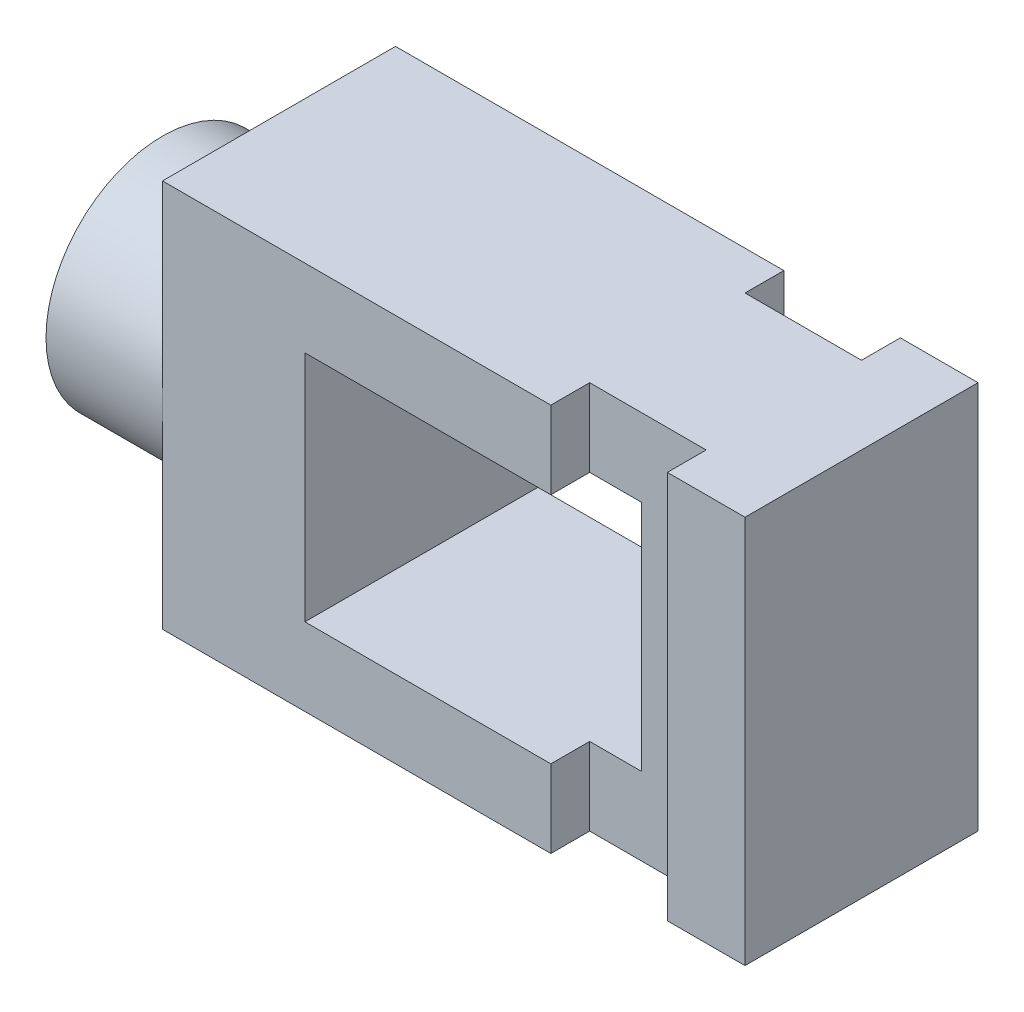
ISO-10303-21;
HEADER;
FILE_DESCRIPTION(('STEP AP214'),'2;1');
FILE_NAME('part.step','',(''),(''),'','','');
FILE_SCHEMA(('AUTOMOTIVE_DESIGN { 1 0 10303 214 1 1 1 1 }'));
ENDSEC;
DATA;
#1=APPLICATION_CONTEXT('core data for automotive mechanical design processes');
#2=APPLICATION_PROTOCOL_DEFINITION('international standard','automotive_design',2000,#1);
#3=PRODUCT_CONTEXT('',#1,'mechanical');
#4=PRODUCT('Part','Part','',(#3));
#5=PRODUCT_RELATED_PRODUCT_CATEGORY('part','',(#4));
#6=PRODUCT_DEFINITION_FORMATION('','',#4);
#7=PRODUCT_DEFINITION_CONTEXT('part definition',#1,'design');
#8=PRODUCT_DEFINITION('design','',#6,#7);
#9=PRODUCT_DEFINITION_SHAPE('','',#8);
#10=(LENGTH_UNIT() NAMED_UNIT(*) SI_UNIT(.MILLI.,.METRE.));
#11=(NAMED_UNIT(*) PLANE_ANGLE_UNIT() SI_UNIT($,.RADIAN.));
#12=(NAMED_UNIT(*) SI_UNIT($,.STERADIAN.) SOLID_ANGLE_UNIT());
#13=UNCERTAINTY_MEASURE_WITH_UNIT(LENGTH_MEASURE(1.E-05),#10,'distance_accuracy_value','');
#14=(GEOMETRIC_REPRESENTATION_CONTEXT(3) GLOBAL_UNCERTAINTY_ASSIGNED_CONTEXT((#13)) GLOBAL_UNIT_ASSIGNED_CONTEXT((#10,
#11,#12)) REPRESENTATION_CONTEXT('',''));
#15=CARTESIAN_POINT('',(0.,0.,0.));
#16=DIRECTION('',(0.,0.,1.));
#17=DIRECTION('',(1.,0.,0.));
#18=AXIS2_PLACEMENT_3D('',#15,#16,#17);
#19=CARTESIAN_POINT('',(0.,0.,36.));
#20=DIRECTION('',(0.,0.,-1.));
#21=DIRECTION('',(-1.,0.,0.));
#22=AXIS2_PLACEMENT_3D('',#19,#20,#21);
#23=PLANE('',#22);
#24=DIRECTION('',(1.,0.,0.));
#25=VECTOR('',#24,1.);
#26=CARTESIAN_POINT('',(-45.,-30.,36.));
#27=LINE('',#26,#25);
#28=CARTESIAN_POINT('',(-45.,-30.,36.));
#29=VERTEX_POINT('',#28);
#30=CARTESIAN_POINT('',(15.,-30.,36.));
#31=VERTEX_POINT('',#30);
#32=EDGE_CURVE('E314',#29,#31,#27,.T.);
#33=ORIENTED_EDGE('',*,*,#32,.T.);
#34=DIRECTION('',(0.,1.,0.));
#35=VECTOR('',#34,1.);
#36=CARTESIAN_POINT('',(15.,0.,36.));
#37=LINE('',#36,#35);
#38=CARTESIAN_POINT('',(15.,-18.,36.));
#39=VERTEX_POINT('',#38);
#40=EDGE_CURVE('E50',#31,#39,#37,.T.);
#41=ORIENTED_EDGE('',*,*,#40,.T.);
#42=DIRECTION('',(1.,0.,0.));
#43=VECTOR('',#42,1.);
#44=CARTESIAN_POINT('',(-23.,-18.,36.));
#45=LINE('',#44,#43);
#46=CARTESIAN_POINT('',(-23.,-18.,36.));
#47=VERTEX_POINT('',#46);
#48=EDGE_CURVE('E278',#47,#39,#45,.T.);
#49=ORIENTED_EDGE('',*,*,#48,.F.);
#50=DIRECTION('',(0.,-1.,0.));
#51=VECTOR('',#50,1.);
#52=CARTESIAN_POINT('',(-23.,-18.,36.));
#53=LINE('',#52,#51);
#54=CARTESIAN_POINT('',(-23.,18.,36.));
#55=VERTEX_POINT('',#54);
#56=EDGE_CURVE('E288',#55,#47,#53,.T.);
#57=ORIENTED_EDGE('',*,*,#56,.F.);
#58=DIRECTION('',(-1.,0.,0.));
#59=VECTOR('',#58,1.);
#60=CARTESIAN_POINT('',(-23.,18.,36.));
#61=LINE('',#60,#59);
#62=CARTESIAN_POINT('',(15.,18.,36.));
#63=VERTEX_POINT('',#62);
#64=EDGE_CURVE('E271',#63,#55,#61,.T.);
#65=ORIENTED_EDGE('',*,*,#64,.F.);
#66=DIRECTION('',(0.,-1.,0.));
#67=VECTOR('',#66,1.);
#68=CARTESIAN_POINT('',(15.,30.,36.));
#69=LINE('',#68,#67);
#70=CARTESIAN_POINT('',(15.,30.,36.));
#71=VERTEX_POINT('',#70);
#72=EDGE_CURVE('E213',#71,#63,#69,.T.);
#73=ORIENTED_EDGE('',*,*,#72,.F.);
#74=DIRECTION('',(-1.,0.,0.));
#75=VECTOR('',#74,1.);
#76=CARTESIAN_POINT('',(-45.,30.,36.));
#77=LINE('',#76,#75);
#78=CARTESIAN_POINT('',(-45.,30.,36.));
#79=VERTEX_POINT('',#78);
#80=EDGE_CURVE('E204',#71,#79,#77,.T.);
#81=ORIENTED_EDGE('',*,*,#80,.T.);
#82=DIRECTION('',(0.,-1.,0.));
#83=VECTOR('',#82,1.);
#84=CARTESIAN_POINT('',(-45.,-30.,36.));
#85=LINE('',#84,#83);
#86=CARTESIAN_POINT('',(-45.,0.,36.));
#87=VERTEX_POINT('',#86);
#88=EDGE_CURVE('E315',#79,#87,#85,.T.);
#89=ORIENTED_EDGE('',*,*,#88,.T.);
#90=EDGE_CURVE('E311',#87,#29,#85,.T.);
#91=ORIENTED_EDGE('',*,*,#90,.T.);
#92=EDGE_LOOP('',(#33,#41,#49,#57,#65,#73,#81,#89,#91));
#93=FACE_BOUND('',#92,.T.);
#94=ADVANCED_FACE('F39',(#93),#23,.F.);
#95=CARTESIAN_POINT('',(-45.,30.,36.));
#96=DIRECTION('',(0.,-1.,0.));
#97=DIRECTION('',(0.,0.,-1.));
#98=AXIS2_PLACEMENT_3D('',#95,#96,#97);
#99=PLANE('',#98);
#100=ORIENTED_EDGE('',*,*,#80,.F.);
#101=DIRECTION('',(0.,0.,-1.));
#102=VECTOR('',#101,1.);
#103=CARTESIAN_POINT('',(15.,30.,36.));
#104=LINE('',#103,#102);
#105=CARTESIAN_POINT('',(15.,30.,30.));
#106=VERTEX_POINT('',#105);
#107=EDGE_CURVE('E184',#71,#106,#104,.T.);
#108=ORIENTED_EDGE('',*,*,#107,.T.);
#109=DIRECTION('',(1.,0.,0.));
#110=VECTOR('',#109,1.);
#111=CARTESIAN_POINT('',(15.,30.,30.));
#112=LINE('',#111,#110);
#113=CARTESIAN_POINT('',(33.,30.,30.));
#114=VERTEX_POINT('',#113);
#115=EDGE_CURVE('E191',#106,#114,#112,.T.);
#116=ORIENTED_EDGE('',*,*,#115,.T.);
#117=DIRECTION('',(0.,0.,1.));
#118=VECTOR('',#117,1.);
#119=CARTESIAN_POINT('',(33.,30.,36.));
#120=LINE('',#119,#118);
#121=CARTESIAN_POINT('',(33.,30.,36.));
#122=VERTEX_POINT('',#121);
#123=EDGE_CURVE('E197',#114,#122,#120,.T.);
#124=ORIENTED_EDGE('',*,*,#123,.T.);
#125=CARTESIAN_POINT('',(45.,30.,36.));
#126=VERTEX_POINT('',#125);
#127=EDGE_CURVE('E308',#126,#122,#77,.T.);
#128=ORIENTED_EDGE('',*,*,#127,.F.);
#129=DIRECTION('',(0.,0.,-1.));
#130=VECTOR('',#129,1.);
#131=CARTESIAN_POINT('',(45.,30.,36.));
#132=LINE('',#131,#130);
#133=CARTESIAN_POINT('',(45.,30.,0.));
#134=VERTEX_POINT('',#133);
#135=EDGE_CURVE('E338',#126,#134,#132,.T.);
#136=ORIENTED_EDGE('',*,*,#135,.T.);
#137=DIRECTION('',(-1.,0.,0.));
#138=VECTOR('',#137,1.);
#139=CARTESIAN_POINT('',(-45.,30.,0.));
#140=LINE('',#139,#138);
#141=CARTESIAN_POINT('',(33.,30.,0.));
#142=VERTEX_POINT('',#141);
#143=EDGE_CURVE('E325',#134,#142,#140,.T.);
#144=ORIENTED_EDGE('',*,*,#143,.T.);
#145=DIRECTION('',(0.,0.,1.));
#146=VECTOR('',#145,1.);
#147=CARTESIAN_POINT('',(33.,30.,0.));
#148=LINE('',#147,#146);
#149=CARTESIAN_POINT('',(33.,30.,6.));
#150=VERTEX_POINT('',#149);
#151=EDGE_CURVE('E233',#142,#150,#148,.T.);
#152=ORIENTED_EDGE('',*,*,#151,.T.);
#153=DIRECTION('',(1.,0.,0.));
#154=VECTOR('',#153,1.);
#155=CARTESIAN_POINT('',(0.,30.,6.));
#156=LINE('',#155,#154);
#157=CARTESIAN_POINT('',(15.,30.,6.));
#158=VERTEX_POINT('',#157);
#159=EDGE_CURVE('E234',#158,#150,#156,.T.);
#160=ORIENTED_EDGE('',*,*,#159,.F.);
#161=DIRECTION('',(0.,0.,1.));
#162=VECTOR('',#161,1.);
#163=CARTESIAN_POINT('',(15.,30.,0.));
#164=LINE('',#163,#162);
#165=CARTESIAN_POINT('',(15.,30.,0.));
#166=VERTEX_POINT('',#165);
#167=EDGE_CURVE('E240',#166,#158,#164,.T.);
#168=ORIENTED_EDGE('',*,*,#167,.F.);
#169=CARTESIAN_POINT('',(-45.,30.,0.));
#170=VERTEX_POINT('',#169);
#171=EDGE_CURVE('E322',#166,#170,#140,.T.);
#172=ORIENTED_EDGE('',*,*,#171,.T.);
#173=DIRECTION('',(0.,0.,-1.));
#174=VECTOR('',#173,1.);
#175=CARTESIAN_POINT('',(-45.,30.,36.));
#176=LINE('',#175,#174);
#177=EDGE_CURVE('E340',#79,#170,#176,.T.);
#178=ORIENTED_EDGE('',*,*,#177,.F.);
#179=EDGE_LOOP('',(#100,#108,#116,#124,#128,#136,#144,#152,#160,#168,#172,#178));
#180=FACE_BOUND('',#179,.T.);
#181=ADVANCED_FACE('F203',(#180),#99,.F.);
#182=CARTESIAN_POINT('',(-45.,-30.,36.));
#183=DIRECTION('',(0.,1.,0.));
#184=DIRECTION('',(0.,0.,1.));
#185=AXIS2_PLACEMENT_3D('',#182,#183,#184);
#186=PLANE('',#185);
#187=DIRECTION('',(1.,0.,0.));
#188=VECTOR('',#187,1.);
#189=CARTESIAN_POINT('',(15.,-30.,30.));
#190=LINE('',#189,#188);
#191=CARTESIAN_POINT('',(15.,-30.,30.));
#192=VERTEX_POINT('',#191);
#193=CARTESIAN_POINT('',(33.,-30.,30.));
#194=VERTEX_POINT('',#193);
#195=EDGE_CURVE('E210',#192,#194,#190,.T.);
#196=ORIENTED_EDGE('',*,*,#195,.F.);
#197=DIRECTION('',(0.,0.,-1.));
#198=VECTOR('',#197,1.);
#199=CARTESIAN_POINT('',(15.,-30.,36.));
#200=LINE('',#199,#198);
#201=EDGE_CURVE('E212',#31,#192,#200,.T.);
#202=ORIENTED_EDGE('',*,*,#201,.F.);
#203=ORIENTED_EDGE('',*,*,#32,.F.);
#204=DIRECTION('',(0.,0.,-1.));
#205=VECTOR('',#204,1.);
#206=CARTESIAN_POINT('',(-45.,-30.,36.));
#207=LINE('',#206,#205);
#208=CARTESIAN_POINT('',(-45.,-30.,0.));
#209=VERTEX_POINT('',#208);
#210=EDGE_CURVE('E332',#29,#209,#207,.T.);
#211=ORIENTED_EDGE('',*,*,#210,.T.);
#212=DIRECTION('',(1.,0.,0.));
#213=VECTOR('',#212,1.);
#214=CARTESIAN_POINT('',(-45.,-30.,0.));
#215=LINE('',#214,#213);
#216=CARTESIAN_POINT('',(15.,-30.,0.));
#217=VERTEX_POINT('',#216);
#218=EDGE_CURVE('E310',#209,#217,#215,.T.);
#219=ORIENTED_EDGE('',*,*,#218,.T.);
#220=DIRECTION('',(0.,0.,1.));
#221=VECTOR('',#220,1.);
#222=CARTESIAN_POINT('',(15.,-30.,0.));
#223=LINE('',#222,#221);
#224=CARTESIAN_POINT('',(15.,-30.,6.));
#225=VERTEX_POINT('',#224);
#226=EDGE_CURVE('E232',#217,#225,#223,.T.);
#227=ORIENTED_EDGE('',*,*,#226,.T.);
#228=DIRECTION('',(1.,0.,0.));
#229=VECTOR('',#228,1.);
#230=CARTESIAN_POINT('',(0.,-30.,6.));
#231=LINE('',#230,#229);
#232=CARTESIAN_POINT('',(33.,-30.,6.));
#233=VERTEX_POINT('',#232);
#234=EDGE_CURVE('E245',#225,#233,#231,.T.);
#235=ORIENTED_EDGE('',*,*,#234,.T.);
#236=DIRECTION('',(0.,0.,1.));
#237=VECTOR('',#236,1.);
#238=CARTESIAN_POINT('',(33.,-30.,0.));
#239=LINE('',#238,#237);
#240=CARTESIAN_POINT('',(33.,-30.,0.));
#241=VERTEX_POINT('',#240);
#242=EDGE_CURVE('E229',#241,#233,#239,.T.);
#243=ORIENTED_EDGE('',*,*,#242,.F.);
#244=CARTESIAN_POINT('',(45.,-30.,0.));
#245=VERTEX_POINT('',#244);
#246=EDGE_CURVE('E329',#241,#245,#215,.T.);
#247=ORIENTED_EDGE('',*,*,#246,.T.);
#248=DIRECTION('',(0.,0.,-1.));
#249=VECTOR('',#248,1.);
#250=CARTESIAN_POINT('',(45.,-30.,36.));
#251=LINE('',#250,#249);
#252=CARTESIAN_POINT('',(45.,-30.,36.));
#253=VERTEX_POINT('',#252);
#254=EDGE_CURVE('E319',#253,#245,#251,.T.);
#255=ORIENTED_EDGE('',*,*,#254,.F.);
#256=CARTESIAN_POINT('',(33.,-30.,36.));
#257=VERTEX_POINT('',#256);
#258=EDGE_CURVE('E313',#257,#253,#27,.T.);
#259=ORIENTED_EDGE('',*,*,#258,.F.);
#260=DIRECTION('',(0.,0.,1.));
#261=VECTOR('',#260,1.);
#262=CARTESIAN_POINT('',(33.,-30.,36.));
#263=LINE('',#262,#261);
#264=EDGE_CURVE('E53',#194,#257,#263,.T.);
#265=ORIENTED_EDGE('',*,*,#264,.F.);
#266=EDGE_LOOP('',(#196,#202,#203,#211,#219,#227,#235,#243,#247,#255,#259,#265));
#267=FACE_BOUND('',#266,.T.);
#268=ADVANCED_FACE('F372',(#267),#186,.F.);
#269=CARTESIAN_POINT('',(0.,0.,0.));
#270=DIRECTION('',(0.,0.,-1.));
#271=DIRECTION('',(-1.,0.,0.));
#272=AXIS2_PLACEMENT_3D('',#269,#270,#271);
#273=PLANE('',#272);
#274=ORIENTED_EDGE('',*,*,#171,.F.);
#275=DIRECTION('',(0.,-1.,0.));
#276=VECTOR('',#275,1.);
#277=CARTESIAN_POINT('',(15.,30.,0.));
#278=LINE('',#277,#276);
#279=CARTESIAN_POINT('',(15.,18.,0.));
#280=VERTEX_POINT('',#279);
#281=EDGE_CURVE('E250',#166,#280,#278,.T.);
#282=ORIENTED_EDGE('',*,*,#281,.T.);
#283=DIRECTION('',(-1.,0.,0.));
#284=VECTOR('',#283,1.);
#285=CARTESIAN_POINT('',(-23.,18.,0.));
#286=LINE('',#285,#284);
#287=CARTESIAN_POINT('',(-23.,18.,0.));
#288=VERTEX_POINT('',#287);
#289=EDGE_CURVE('E280',#280,#288,#286,.T.);
#290=ORIENTED_EDGE('',*,*,#289,.T.);
#291=DIRECTION('',(0.,-1.,0.));
#292=VECTOR('',#291,1.);
#293=CARTESIAN_POINT('',(-23.,-18.,0.));
#294=LINE('',#293,#292);
#295=CARTESIAN_POINT('',(-23.,-18.,0.));
#296=VERTEX_POINT('',#295);
#297=EDGE_CURVE('E276',#288,#296,#294,.T.);
#298=ORIENTED_EDGE('',*,*,#297,.T.);
#299=DIRECTION('',(1.,0.,0.));
#300=VECTOR('',#299,1.);
#301=CARTESIAN_POINT('',(-23.,-18.,0.));
#302=LINE('',#301,#300);
#303=CARTESIAN_POINT('',(15.,-18.,0.));
#304=VERTEX_POINT('',#303);
#305=EDGE_CURVE('E281',#296,#304,#302,.T.);
#306=ORIENTED_EDGE('',*,*,#305,.T.);
#307=EDGE_CURVE('E249',#304,#217,#278,.T.);
#308=ORIENTED_EDGE('',*,*,#307,.T.);
#309=ORIENTED_EDGE('',*,*,#218,.F.);
#310=DIRECTION('',(0.,-1.,0.));
#311=VECTOR('',#310,1.);
#312=CARTESIAN_POINT('',(-45.,-30.,0.));
#313=LINE('',#312,#311);
#314=CARTESIAN_POINT('',(-45.,0.,0.));
#315=VERTEX_POINT('',#314);
#316=EDGE_CURVE('E323',#315,#209,#313,.T.);
#317=ORIENTED_EDGE('',*,*,#316,.F.);
#318=EDGE_CURVE('E328',#170,#315,#313,.T.);
#319=ORIENTED_EDGE('',*,*,#318,.F.);
#320=EDGE_LOOP('',(#274,#282,#290,#298,#306,#308,#309,#317,#319));
#321=FACE_BOUND('',#320,.T.);
#322=ADVANCED_FACE('F405',(#321),#273,.T.);
#323=CARTESIAN_POINT('',(23.,-18.,0.));
#324=DIRECTION('',(1.,0.,0.));
#325=DIRECTION('',(0.,0.,-1.));
#326=AXIS2_PLACEMENT_3D('',#323,#324,#325);
#327=PLANE('',#326);
#328=DIRECTION('',(0.,0.,1.));
#329=VECTOR('',#328,1.);
#330=CARTESIAN_POINT('',(23.,-18.,0.));
#331=LINE('',#330,#329);
#332=CARTESIAN_POINT('',(23.,-18.,6.));
#333=VERTEX_POINT('',#332);
#334=CARTESIAN_POINT('',(23.,-18.,30.));
#335=VERTEX_POINT('',#334);
#336=EDGE_CURVE('E291',#333,#335,#331,.T.);
#337=ORIENTED_EDGE('',*,*,#336,.T.);
#338=DIRECTION('',(0.,1.,0.));
#339=VECTOR('',#338,1.);
#340=CARTESIAN_POINT('',(23.,-18.,30.));
#341=LINE('',#340,#339);
#342=CARTESIAN_POINT('',(23.,18.,30.));
#343=VERTEX_POINT('',#342);
#344=EDGE_CURVE('E222',#335,#343,#341,.T.);
#345=ORIENTED_EDGE('',*,*,#344,.T.);
#346=DIRECTION('',(0.,0.,1.));
#347=VECTOR('',#346,1.);
#348=CARTESIAN_POINT('',(23.,18.,0.));
#349=LINE('',#348,#347);
#350=CARTESIAN_POINT('',(23.,18.,6.));
#351=VERTEX_POINT('',#350);
#352=EDGE_CURVE('E286',#351,#343,#349,.T.);
#353=ORIENTED_EDGE('',*,*,#352,.F.);
#354=DIRECTION('',(0.,1.,0.));
#355=VECTOR('',#354,1.);
#356=CARTESIAN_POINT('',(23.,-18.,6.));
#357=LINE('',#356,#355);
#358=EDGE_CURVE('E65',#333,#351,#357,.T.);
#359=ORIENTED_EDGE('',*,*,#358,.F.);
#360=EDGE_LOOP('',(#337,#345,#353,#359));
#361=FACE_BOUND('',#360,.T.);
#362=ADVANCED_FACE('F370',(#361),#327,.F.);
#363=CARTESIAN_POINT('',(-23.,-18.,0.));
#364=DIRECTION('',(0.,-1.,0.));
#365=DIRECTION('',(0.,0.,-1.));
#366=AXIS2_PLACEMENT_3D('',#363,#364,#365);
#367=PLANE('',#366);
#368=ORIENTED_EDGE('',*,*,#48,.T.);
#369=DIRECTION('',(0.,0.,-1.));
#370=VECTOR('',#369,1.);
#371=CARTESIAN_POINT('',(15.,-18.,0.));
#372=LINE('',#371,#370);
#373=CARTESIAN_POINT('',(15.,-18.,30.));
#374=VERTEX_POINT('',#373);
#375=EDGE_CURVE('E221',#39,#374,#372,.T.);
#376=ORIENTED_EDGE('',*,*,#375,.T.);
#377=DIRECTION('',(1.,0.,0.));
#378=VECTOR('',#377,1.);
#379=CARTESIAN_POINT('',(-23.,-18.,30.));
#380=LINE('',#379,#378);
#381=EDGE_CURVE('E227',#374,#335,#380,.T.);
#382=ORIENTED_EDGE('',*,*,#381,.T.);
#383=ORIENTED_EDGE('',*,*,#336,.F.);
#384=DIRECTION('',(1.,0.,0.));
#385=VECTOR('',#384,1.);
#386=CARTESIAN_POINT('',(-23.,-18.,6.));
#387=LINE('',#386,#385);
#388=CARTESIAN_POINT('',(15.,-18.,6.));
#389=VERTEX_POINT('',#388);
#390=EDGE_CURVE('E256',#389,#333,#387,.T.);
#391=ORIENTED_EDGE('',*,*,#390,.F.);
#392=DIRECTION('',(0.,0.,1.));
#393=VECTOR('',#392,1.);
#394=CARTESIAN_POINT('',(15.,-18.,0.));
#395=LINE('',#394,#393);
#396=EDGE_CURVE('E263',#304,#389,#395,.T.);
#397=ORIENTED_EDGE('',*,*,#396,.F.);
#398=ORIENTED_EDGE('',*,*,#305,.F.);
#399=DIRECTION('',(0.,0.,1.));
#400=VECTOR('',#399,1.);
#401=CARTESIAN_POINT('',(-23.,-18.,0.));
#402=LINE('',#401,#400);
#403=EDGE_CURVE('E300',#296,#47,#402,.T.);
#404=ORIENTED_EDGE('',*,*,#403,.T.);
#405=EDGE_LOOP('',(#368,#376,#382,#383,#391,#397,#398,#404));
#406=FACE_BOUND('',#405,.T.);
#407=ADVANCED_FACE('F352',(#406),#367,.F.);
#408=CARTESIAN_POINT('',(-23.,18.,0.));
#409=DIRECTION('',(0.,1.,0.));
#410=DIRECTION('',(0.,0.,1.));
#411=AXIS2_PLACEMENT_3D('',#408,#409,#410);
#412=PLANE('',#411);
#413=DIRECTION('',(-1.,0.,0.));
#414=VECTOR('',#413,1.);
#415=CARTESIAN_POINT('',(-23.,18.,30.));
#416=LINE('',#415,#414);
#417=CARTESIAN_POINT('',(15.,18.,30.));
#418=VERTEX_POINT('',#417);
#419=EDGE_CURVE('E11',#343,#418,#416,.T.);
#420=ORIENTED_EDGE('',*,*,#419,.T.);
#421=DIRECTION('',(0.,0.,1.));
#422=VECTOR('',#421,1.);
#423=CARTESIAN_POINT('',(15.,18.,0.));
#424=LINE('',#423,#422);
#425=EDGE_CURVE('E189',#418,#63,#424,.T.);
#426=ORIENTED_EDGE('',*,*,#425,.T.);
#427=ORIENTED_EDGE('',*,*,#64,.T.);
#428=DIRECTION('',(0.,0.,1.));
#429=VECTOR('',#428,1.);
#430=CARTESIAN_POINT('',(-23.,18.,0.));
#431=LINE('',#430,#429);
#432=EDGE_CURVE('E299',#288,#55,#431,.T.);
#433=ORIENTED_EDGE('',*,*,#432,.F.);
#434=ORIENTED_EDGE('',*,*,#289,.F.);
#435=DIRECTION('',(0.,0.,-1.));
#436=VECTOR('',#435,1.);
#437=CARTESIAN_POINT('',(15.,18.,0.));
#438=LINE('',#437,#436);
#439=CARTESIAN_POINT('',(15.,18.,6.));
#440=VERTEX_POINT('',#439);
#441=EDGE_CURVE('E343',#440,#280,#438,.T.);
#442=ORIENTED_EDGE('',*,*,#441,.F.);
#443=DIRECTION('',(-1.,0.,0.));
#444=VECTOR('',#443,1.);
#445=CARTESIAN_POINT('',(-23.,18.,6.));
#446=LINE('',#445,#444);
#447=EDGE_CURVE('E344',#351,#440,#446,.T.);
#448=ORIENTED_EDGE('',*,*,#447,.F.);
#449=ORIENTED_EDGE('',*,*,#352,.T.);
#450=EDGE_LOOP('',(#420,#426,#427,#433,#434,#442,#448,#449));
#451=FACE_BOUND('',#450,.T.);
#452=ADVANCED_FACE('F361',(#451),#412,.F.);
#453=CARTESIAN_POINT('',(-45.,-30.,36.));
#454=DIRECTION('',(1.,0.,0.));
#455=DIRECTION('',(0.,0.,-1.));
#456=AXIS2_PLACEMENT_3D('',#453,#454,#455);
#457=PLANE('',#456);
#458=CARTESIAN_POINT('',(-45.,0.,18.));
#459=DIRECTION('',(-1.,0.,0.));
#460=DIRECTION('',(0.,0.,1.));
#461=AXIS2_PLACEMENT_3D('',#458,#459,#460);
#462=CIRCLE('',#461,18.);
#463=EDGE_CURVE('E270',#87,#315,#462,.T.);
#464=ORIENTED_EDGE('',*,*,#463,.F.);
#465=ORIENTED_EDGE('',*,*,#88,.F.);
#466=ORIENTED_EDGE('',*,*,#177,.T.);
#467=ORIENTED_EDGE('',*,*,#318,.T.);
#468=EDGE_LOOP('',(#464,#465,#466,#467));
#469=FACE_BOUND('',#468,.T.);
#470=ADVANCED_FACE('F410',(#469),#457,.F.);
#471=CARTESIAN_POINT('',(45.,-30.,36.));
#472=DIRECTION('',(-1.,0.,0.));
#473=DIRECTION('',(0.,0.,1.));
#474=AXIS2_PLACEMENT_3D('',#471,#472,#473);
#475=PLANE('',#474);
#476=DIRECTION('',(0.,1.,0.));
#477=VECTOR('',#476,1.);
#478=CARTESIAN_POINT('',(45.,-30.,0.));
#479=LINE('',#478,#477);
#480=EDGE_CURVE('E298',#245,#134,#479,.T.);
#481=ORIENTED_EDGE('',*,*,#480,.T.);
#482=ORIENTED_EDGE('',*,*,#135,.F.);
#483=DIRECTION('',(0.,1.,0.));
#484=VECTOR('',#483,1.);
#485=CARTESIAN_POINT('',(45.,-30.,36.));
#486=LINE('',#485,#484);
#487=EDGE_CURVE('E302',#253,#126,#486,.T.);
#488=ORIENTED_EDGE('',*,*,#487,.F.);
#489=ORIENTED_EDGE('',*,*,#254,.T.);
#490=EDGE_LOOP('',(#481,#482,#488,#489));
#491=FACE_BOUND('',#490,.T.);
#492=ADVANCED_FACE('F41',(#491),#475,.F.);
#493=EDGE_CURVE('E277',#315,#87,#462,.T.);
#494=ORIENTED_EDGE('',*,*,#493,.F.);
#495=ORIENTED_EDGE('',*,*,#316,.T.);
#496=ORIENTED_EDGE('',*,*,#210,.F.);
#497=ORIENTED_EDGE('',*,*,#90,.F.);
#498=EDGE_LOOP('',(#494,#495,#496,#497));
#499=FACE_BOUND('',#498,.T.);
#500=ADVANCED_FACE('F414',(#499),#457,.F.);
#501=ORIENTED_EDGE('',*,*,#127,.T.);
#502=DIRECTION('',(0.,-1.,0.));
#503=VECTOR('',#502,1.);
#504=CARTESIAN_POINT('',(33.,30.,36.));
#505=LINE('',#504,#503);
#506=EDGE_CURVE('E220',#122,#257,#505,.T.);
#507=ORIENTED_EDGE('',*,*,#506,.T.);
#508=ORIENTED_EDGE('',*,*,#258,.T.);
#509=ORIENTED_EDGE('',*,*,#487,.T.);
#510=EDGE_LOOP('',(#501,#507,#508,#509));
#511=FACE_BOUND('',#510,.T.);
#512=ADVANCED_FACE('F378',(#511),#23,.F.);
#513=DIRECTION('',(0.,-1.,0.));
#514=VECTOR('',#513,1.);
#515=CARTESIAN_POINT('',(33.,30.,0.));
#516=LINE('',#515,#514);
#517=EDGE_CURVE('E237',#142,#241,#516,.T.);
#518=ORIENTED_EDGE('',*,*,#517,.F.);
#519=ORIENTED_EDGE('',*,*,#143,.F.);
#520=ORIENTED_EDGE('',*,*,#480,.F.);
#521=ORIENTED_EDGE('',*,*,#246,.F.);
#522=EDGE_LOOP('',(#518,#519,#520,#521));
#523=FACE_BOUND('',#522,.T.);
#524=ADVANCED_FACE('F390',(#523),#273,.T.);
#525=CARTESIAN_POINT('',(-23.,-18.,0.));
#526=DIRECTION('',(-1.,0.,0.));
#527=DIRECTION('',(0.,0.,1.));
#528=AXIS2_PLACEMENT_3D('',#525,#526,#527);
#529=PLANE('',#528);
#530=ORIENTED_EDGE('',*,*,#56,.T.);
#531=ORIENTED_EDGE('',*,*,#403,.F.);
#532=ORIENTED_EDGE('',*,*,#297,.F.);
#533=ORIENTED_EDGE('',*,*,#432,.T.);
#534=EDGE_LOOP('',(#530,#531,#532,#533));
#535=FACE_BOUND('',#534,.T.);
#536=ADVANCED_FACE('F360',(#535),#529,.F.);
#537=CARTESIAN_POINT('',(-63.,0.,18.));
#538=DIRECTION('',(1.,0.,0.));
#539=DIRECTION('',(0.,0.,-1.));
#540=AXIS2_PLACEMENT_3D('',#537,#538,#539);
#541=CYLINDRICAL_SURFACE('',#540,18.);
#542=CARTESIAN_POINT('',(-63.,0.,18.));
#543=DIRECTION('',(-1.,0.,0.));
#544=DIRECTION('',(0.,0.,1.));
#545=AXIS2_PLACEMENT_3D('',#542,#543,#544);
#546=CIRCLE('',#545,18.);
#547=CARTESIAN_POINT('',(-63.,0.,36.));
#548=VERTEX_POINT('',#547);
#549=EDGE_CURVE('E269',#548,#548,#546,.T.);
#550=ORIENTED_EDGE('',*,*,#549,.F.);
#551=EDGE_LOOP('',(#550));
#552=FACE_BOUND('',#551,.T.);
#553=ORIENTED_EDGE('',*,*,#463,.T.);
#554=ORIENTED_EDGE('',*,*,#493,.T.);
#555=EDGE_LOOP('',(#553,#554));
#556=FACE_BOUND('',#555,.T.);
#557=ADVANCED_FACE('F413',(#552,#556),#541,.T.);
#558=CARTESIAN_POINT('',(-63.,0.,18.));
#559=DIRECTION('',(-1.,0.,0.));
#560=DIRECTION('',(0.,0.,1.));
#561=AXIS2_PLACEMENT_3D('',#558,#559,#560);
#562=PLANE('',#561);
#563=CARTESIAN_POINT('',(-63.,0.,18.));
#564=DIRECTION('',(-1.,0.,0.));
#565=DIRECTION('',(0.,0.,1.));
#566=AXIS2_PLACEMENT_3D('',#563,#564,#565);
#567=CIRCLE('',#566,5.);
#568=CARTESIAN_POINT('',(-63.,0.,23.));
#569=VERTEX_POINT('',#568);
#570=EDGE_CURVE('E261',#569,#569,#567,.T.);
#571=ORIENTED_EDGE('',*,*,#570,.F.);
#572=EDGE_LOOP('',(#571));
#573=FACE_BOUND('',#572,.T.);
#574=ORIENTED_EDGE('',*,*,#549,.T.);
#575=EDGE_LOOP('',(#574));
#576=FACE_BOUND('',#575,.T.);
#577=ADVANCED_FACE('F543',(#573,#576),#562,.T.);
#578=CARTESIAN_POINT('',(-45.,0.,18.));
#579=DIRECTION('',(-1.,0.,0.));
#580=DIRECTION('',(0.,0.,1.));
#581=AXIS2_PLACEMENT_3D('',#578,#579,#580);
#582=CYLINDRICAL_SURFACE('',#581,5.);
#583=CARTESIAN_POINT('',(-45.,0.,18.));
#584=DIRECTION('',(-1.,0.,0.));
#585=DIRECTION('',(0.,0.,1.));
#586=AXIS2_PLACEMENT_3D('',#583,#584,#585);
#587=CIRCLE('',#586,5.);
#588=CARTESIAN_POINT('',(-45.,0.,23.));
#589=VERTEX_POINT('',#588);
#590=EDGE_CURVE('E264',#589,#589,#587,.T.);
#591=ORIENTED_EDGE('',*,*,#590,.F.);
#592=EDGE_LOOP('',(#591));
#593=FACE_BOUND('',#592,.T.);
#594=ORIENTED_EDGE('',*,*,#570,.T.);
#595=EDGE_LOOP('',(#594));
#596=FACE_BOUND('',#595,.T.);
#597=ADVANCED_FACE('F426',(#593,#596),#582,.F.);
#598=CARTESIAN_POINT('',(-45.,0.,18.));
#599=DIRECTION('',(-1.,0.,0.));
#600=DIRECTION('',(0.,0.,1.));
#601=AXIS2_PLACEMENT_3D('',#598,#599,#600);
#602=PLANE('',#601);
#603=ORIENTED_EDGE('',*,*,#590,.T.);
#604=EDGE_LOOP('',(#603));
#605=FACE_BOUND('',#604,.T.);
#606=ADVANCED_FACE('F423',(#605),#602,.T.);
#607=CARTESIAN_POINT('',(15.,30.,0.));
#608=DIRECTION('',(1.,0.,0.));
#609=DIRECTION('',(0.,0.,-1.));
#610=AXIS2_PLACEMENT_3D('',#607,#608,#609);
#611=PLANE('',#610);
#612=ORIENTED_EDGE('',*,*,#396,.T.);
#613=DIRECTION('',(0.,-1.,0.));
#614=VECTOR('',#613,1.);
#615=CARTESIAN_POINT('',(15.,30.,6.));
#616=LINE('',#615,#614);
#617=EDGE_CURVE('E251',#389,#225,#616,.T.);
#618=ORIENTED_EDGE('',*,*,#617,.T.);
#619=ORIENTED_EDGE('',*,*,#226,.F.);
#620=ORIENTED_EDGE('',*,*,#307,.F.);
#621=EDGE_LOOP('',(#612,#618,#619,#620));
#622=FACE_BOUND('',#621,.T.);
#623=ADVANCED_FACE('F418',(#622),#611,.T.);
#624=ORIENTED_EDGE('',*,*,#441,.T.);
#625=ORIENTED_EDGE('',*,*,#281,.F.);
#626=ORIENTED_EDGE('',*,*,#167,.T.);
#627=EDGE_CURVE('E252',#158,#440,#616,.T.);
#628=ORIENTED_EDGE('',*,*,#627,.T.);
#629=EDGE_LOOP('',(#624,#625,#626,#628));
#630=FACE_BOUND('',#629,.T.);
#631=ADVANCED_FACE('F419',(#630),#611,.T.);
#632=CARTESIAN_POINT('',(0.,30.,6.));
#633=DIRECTION('',(0.,0.,-1.));
#634=DIRECTION('',(-1.,0.,0.));
#635=AXIS2_PLACEMENT_3D('',#632,#633,#634);
#636=PLANE('',#635);
#637=ORIENTED_EDGE('',*,*,#390,.T.);
#638=ORIENTED_EDGE('',*,*,#358,.T.);
#639=ORIENTED_EDGE('',*,*,#447,.T.);
#640=ORIENTED_EDGE('',*,*,#627,.F.);
#641=ORIENTED_EDGE('',*,*,#159,.T.);
#642=DIRECTION('',(0.,-1.,0.));
#643=VECTOR('',#642,1.);
#644=CARTESIAN_POINT('',(33.,30.,6.));
#645=LINE('',#644,#643);
#646=EDGE_CURVE('E253',#150,#233,#645,.T.);
#647=ORIENTED_EDGE('',*,*,#646,.T.);
#648=ORIENTED_EDGE('',*,*,#234,.F.);
#649=ORIENTED_EDGE('',*,*,#617,.F.);
#650=EDGE_LOOP('',(#637,#638,#639,#640,#641,#647,#648,#649));
#651=FACE_BOUND('',#650,.T.);
#652=ADVANCED_FACE('F394',(#651),#636,.T.);
#653=CARTESIAN_POINT('',(33.,30.,0.));
#654=DIRECTION('',(1.,0.,0.));
#655=DIRECTION('',(0.,0.,-1.));
#656=AXIS2_PLACEMENT_3D('',#653,#654,#655);
#657=PLANE('',#656);
#658=ORIENTED_EDGE('',*,*,#242,.T.);
#659=ORIENTED_EDGE('',*,*,#646,.F.);
#660=ORIENTED_EDGE('',*,*,#151,.F.);
#661=ORIENTED_EDGE('',*,*,#517,.T.);
#662=EDGE_LOOP('',(#658,#659,#660,#661));
#663=FACE_BOUND('',#662,.T.);
#664=ADVANCED_FACE('F388',(#663),#657,.F.);
#665=CARTESIAN_POINT('',(15.,30.,30.));
#666=DIRECTION('',(0.,0.,-1.));
#667=DIRECTION('',(-1.,0.,0.));
#668=AXIS2_PLACEMENT_3D('',#665,#666,#667);
#669=PLANE('',#668);
#670=DIRECTION('',(0.,-1.,0.));
#671=VECTOR('',#670,1.);
#672=CARTESIAN_POINT('',(15.,30.,30.));
#673=LINE('',#672,#671);
#674=EDGE_CURVE('E192',#374,#192,#673,.T.);
#675=ORIENTED_EDGE('',*,*,#674,.T.);
#676=ORIENTED_EDGE('',*,*,#195,.T.);
#677=DIRECTION('',(0.,-1.,0.));
#678=VECTOR('',#677,1.);
#679=CARTESIAN_POINT('',(33.,30.,30.));
#680=LINE('',#679,#678);
#681=EDGE_CURVE('E188',#114,#194,#680,.T.);
#682=ORIENTED_EDGE('',*,*,#681,.F.);
#683=ORIENTED_EDGE('',*,*,#115,.F.);
#684=EDGE_CURVE('E181',#106,#418,#673,.T.);
#685=ORIENTED_EDGE('',*,*,#684,.T.);
#686=ORIENTED_EDGE('',*,*,#419,.F.);
#687=ORIENTED_EDGE('',*,*,#344,.F.);
#688=ORIENTED_EDGE('',*,*,#381,.F.);
#689=EDGE_LOOP('',(#675,#676,#682,#683,#685,#686,#687,#688));
#690=FACE_BOUND('',#689,.T.);
#691=ADVANCED_FACE('F193',(#690),#669,.F.);
#692=CARTESIAN_POINT('',(15.,30.,36.));
#693=DIRECTION('',(-1.,0.,0.));
#694=DIRECTION('',(0.,0.,1.));
#695=AXIS2_PLACEMENT_3D('',#692,#693,#694);
#696=PLANE('',#695);
#697=ORIENTED_EDGE('',*,*,#40,.F.);
#698=ORIENTED_EDGE('',*,*,#201,.T.);
#699=ORIENTED_EDGE('',*,*,#674,.F.);
#700=ORIENTED_EDGE('',*,*,#375,.F.);
#701=EDGE_LOOP('',(#697,#698,#699,#700));
#702=FACE_BOUND('',#701,.T.);
#703=ADVANCED_FACE('F371',(#702),#696,.F.);
#704=ORIENTED_EDGE('',*,*,#684,.F.);
#705=ORIENTED_EDGE('',*,*,#107,.F.);
#706=ORIENTED_EDGE('',*,*,#72,.T.);
#707=ORIENTED_EDGE('',*,*,#425,.F.);
#708=EDGE_LOOP('',(#704,#705,#706,#707));
#709=FACE_BOUND('',#708,.T.);
#710=ADVANCED_FACE('F182',(#709),#696,.F.);
#711=CARTESIAN_POINT('',(33.,30.,36.));
#712=DIRECTION('',(1.,0.,0.));
#713=DIRECTION('',(0.,0.,-1.));
#714=AXIS2_PLACEMENT_3D('',#711,#712,#713);
#715=PLANE('',#714);
#716=ORIENTED_EDGE('',*,*,#264,.T.);
#717=ORIENTED_EDGE('',*,*,#506,.F.);
#718=ORIENTED_EDGE('',*,*,#123,.F.);
#719=ORIENTED_EDGE('',*,*,#681,.T.);
#720=EDGE_LOOP('',(#716,#717,#718,#719));
#721=FACE_BOUND('',#720,.T.);
#722=ADVANCED_FACE('F382',(#721),#715,.F.);
#723=CLOSED_SHELL('',(#94,#181,#268,#322,#362,#407,#452,#470,#492,#500,#512,#524,#536,#557,#577,
#597,#606,#623,#631,#652,#664,#691,#703,#710,#722));
#724=MANIFOLD_SOLID_BREP('B2',#723);
#725=ADVANCED_BREP_SHAPE_REPRESENTATION('',(#18,#724),#14);
#726=SHAPE_DEFINITION_REPRESENTATION(#9,#725);
ENDSEC;
END-ISO-10303-21;
